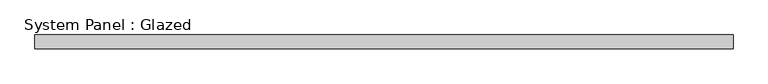
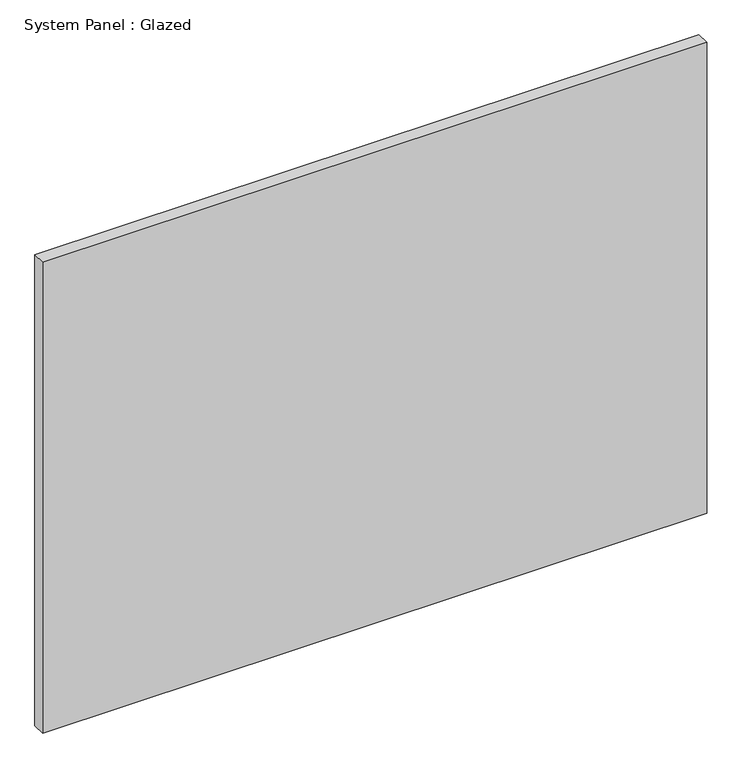
"""IFC4 building model written with IfcOpenShell, lengths in millimetres: plate geometry, System Panel : Glazed."""

from ifc_helpers import new_model, si_unit, origin, origin_with_axes, place, context, project, spatial, polyline, outline, extrude, source, transform, mapped, element, save


def system_panel_glazed_bf93abc5(model_context):
    return source(origin(), model_context, "Body", "SweptSolid", [
        extrude(outline(polyline([(638.175, 19.05), (-638.175, 19.05), (-638.175, 44.45), (638.175, 44.45), (638.175, 19.05)])), origin_with_axes(), (0.0, 0.0, 1.0), 956.453622),
    ])


if __name__ == "__main__":
    model = new_model("IFC4")
    model_context = context("Model", 3, world=origin())
    ifc_project = project(units=[si_unit("LENGTHUNIT", "METRE", prefix="MILLI")], contexts=[model_context])
    site = spatial("IfcSite", under=ifc_project)
    building = spatial("IfcBuilding", under=site)
    placement = place(None, origin())
    system_panel_glazed_shape = system_panel_glazed_bf93abc5(model_context)
    element("IfcPlate", 1, ObjectType="System Panel : Glazed", at=placement, inside=building, context=model_context, shape_type="MappedRepresentation", body=[
        mapped(system_panel_glazed_shape, transform((0.0, 0.0, 0.0), x_axis=(1.0, 0.0, 0.0), y_axis=(0.0, 1.0, 0.0), z_axis=(0.0, 0.0, 1.0))),
    ])
    save(model, "model.ifc")

# Revit data of these elements
# Type "System Panel : Glazed"
#   Construction Type Id = "GSP4R"
#   Analytic Construction = "1/8 in Pilkington single glazing"
#   Visual Light Transmittance = 0.9
#   Solar Heat Gain Coefficient = 0.86
#   Heat Transfer Coefficient (U) = 1.18115 BTU/(h·ft²·°F)
#   Define Thermal Properties by = 1
# Element 1 (IfcPlate, "System Panel : Glazed")
#   Materials on its faces: "Glass"
# Materials
#   "Glass": class "Glass", colour RGB 0 128 192, transparency 0.75, Description = "Soda Lime Glass", Cost = 0
